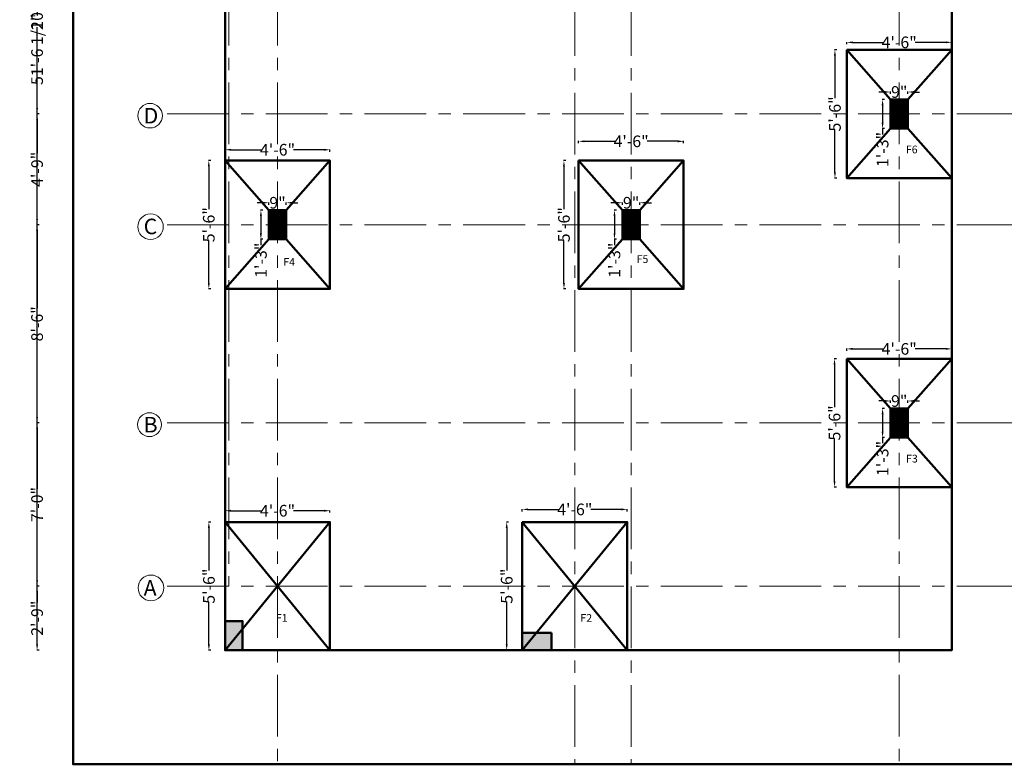
# Model space of a CAD drawing. Units: inches. Extents: x -114 to 953, y -626 to 140.
# Tile 1 of 3: x -114 to 393, y -626 to -243. Entities that reach past the tile are written whole.
import ezdxf

# ---------------------------------------------------------------- set-up
doc = ezdxf.new("R2010")
doc.units = ezdxf.units.IN
doc.header["$MEASUREMENT"] = 0
doc.linetypes.add('CENTER', pattern=[50.8, 31.75, -6.35, 6.35, -6.35])
for name, color, linetype, lineweight in [('S-ANNO-DIMS', 2, 'Continuous', 25), ('S-ANNO-TEXT', 3, 'Continuous', 25), ('S-ANNO-TTLB', 7, 'Continuous', 50), ('S-FNDN', 7, 'Continuous', 50), ('S-FNDN-PATT', 252, 'Continuous', 13), ('S-GRID', 1, 'CENTER', 18), ('S-GRID-IDEN', 7, 'Continuous', 18)]:
    doc.layers.add(name, color=color, linetype=linetype, lineweight=lineweight)
doc.styles.get("Standard").update_dxf_attribs({"font": 'arial.ttf'})
doc.dimstyles.get("Standard").update_dxf_attribs({"dimtxt": 6, "dimasz": 3, "dimexe": 0.18, "dimexo": 0.0625, "dimgap": 0.09, "dimtad": 0, "dimzin": 0, "dimdsep": 46, "dimlunit": 4, "dimtxsty": 'Standard', "dimcen": 0.09, "dimclrd": 256, "dimclrt": 6, "dimadec": 0, "dimazin": 0, "dimtfac": 6, "dimtofl": 0, "dimtmove": 0, "dimatfit": 3, "dimfxl": 1, "dimfxlon": 1, "dimtolj": 1, "dimtzin": 0, "dimarcsym": 0})

# ---------------------------------------------------------------- blocks, each defined once
blk = doc.blocks.new('*D9')
at = {"layer": 'Defpoints', "color": 0, "transparency": 16777216}
for p in [(23.4, -337.38), (14.4, -341.17), (23.4, -341.17)]:
    blk.add_point(p, dxfattribs=at)
at = {"layer": 'S-ANNO-DIMS', "color": 0, "lineweight": -2, "transparency": 16777216}
for p, q in [((11.4, -337.38), (8.4, -337.38)), ((14.4, -338.38), (14.4, -337.2)), ((23.4, -338.38), (23.4, -337.2)), ((26.4, -337.38), (29.4, -337.38))]:
    blk.add_line(p, q, dxfattribs=at)
at = {"layer": 'S-ANNO-DIMS', "color": 0, "transparency": 16777216}
for points in [[(11.4, -336.88), (11.4, -337.88), (14.4, -337.38)], [(26.4, -336.88), (26.4, -337.88), (23.4, -337.38)]]:
    blk.add_solid(points, dxfattribs=at)
at = {"layer": 'S-ANNO-DIMS', "color": 0, "transparency": 16777216, "insert": (18.9, -337.38), "char_height": 6, "attachment_point": 5}
blk.add_mtext('\\A1;9"', dxfattribs=at)
blk = doc.blocks.new('*D10')
at = {"layer": 'Defpoints', "color": 0, "transparency": 16777216}
for p in [(14.4, -341.17), (10.34, -356.17), (14.4, -356.17)]:
    blk.add_point(p, dxfattribs=at)
at = {"layer": 'S-ANNO-DIMS', "color": 0, "lineweight": -2, "transparency": 16777216}
for p, q in [((11.34, -341.17), (10.16, -341.17)), ((10.34, -344.17), (10.34, -353.17)), ((11.34, -356.17), (10.16, -356.17)), ((10.34, -356.17), (10.34, -359.17))]:
    blk.add_line(p, q, dxfattribs=at)
at = {"layer": 'S-ANNO-DIMS', "color": 0, "transparency": 16777216}
for points in [[(9.84, -344.17), (10.84, -344.17), (10.34, -341.17)], [(9.84, -353.17), (10.84, -353.17), (10.34, -356.17)]]:
    blk.add_solid(points, dxfattribs=at)
at = {"layer": 'S-ANNO-DIMS', "color": 0, "transparency": 16777216, "insert": (10.34, -366.95), "char_height": 6, "attachment_point": 5, "rotation": 90}
blk.add_mtext('\\A1;1\'-3"', dxfattribs=at)
blk = doc.blocks.new('*D11')
at = {"layer": 'Defpoints', "color": 0, "transparency": 16777216}
for p in [(343.4, -280.38), (334.4, -284.17), (343.4, -284.17)]:
    blk.add_point(p, dxfattribs=at)
at = {"layer": 'S-ANNO-DIMS', "color": 0, "lineweight": -2, "transparency": 16777216}
for p, q in [((331.4, -280.38), (328.4, -280.38)), ((334.4, -281.38), (334.4, -280.2)), ((343.4, -281.38), (343.4, -280.2)), ((346.4, -280.38), (349.4, -280.38))]:
    blk.add_line(p, q, dxfattribs=at)
at = {"layer": 'S-ANNO-DIMS', "color": 0, "transparency": 16777216}
for points in [[(331.4, -279.88), (331.4, -280.88), (334.4, -280.38)], [(346.4, -279.88), (346.4, -280.88), (343.4, -280.38)]]:
    blk.add_solid(points, dxfattribs=at)
at = {"layer": 'S-ANNO-DIMS', "color": 0, "transparency": 16777216, "insert": (338.9, -280.38), "char_height": 6, "attachment_point": 5}
blk.add_mtext('\\A1;9"', dxfattribs=at)
blk = doc.blocks.new('*D12')
at = {"layer": 'Defpoints', "color": 0, "transparency": 16777216}
for p in [(334.4, -284.17), (330.34, -299.17), (334.4, -299.17)]:
    blk.add_point(p, dxfattribs=at)
at = {"layer": 'S-ANNO-DIMS', "color": 0, "lineweight": -2, "transparency": 16777216}
for p, q in [((331.34, -284.17), (330.16, -284.17)), ((330.34, -287.17), (330.34, -296.17)), ((331.34, -299.17), (330.16, -299.17)), ((330.34, -299.17), (330.34, -302.17))]:
    blk.add_line(p, q, dxfattribs=at)
at = {"layer": 'S-ANNO-DIMS', "color": 0, "transparency": 16777216}
for points in [[(329.84, -287.17), (330.84, -287.17), (330.34, -284.17)], [(329.84, -296.17), (330.84, -296.17), (330.34, -299.17)]]:
    blk.add_solid(points, dxfattribs=at)
at = {"layer": 'S-ANNO-DIMS', "color": 0, "transparency": 16777216, "insert": (330.34, -309.95), "char_height": 6, "attachment_point": 5, "rotation": 90}
blk.add_mtext('\\A1;1\'-3"', dxfattribs=at)
blk = doc.blocks.new('*D13')
at = {"layer": 'Defpoints', "color": 0, "transparency": 16777216}
for p in [(343.4, -439.38), (334.4, -443.17), (343.4, -443.17)]:
    blk.add_point(p, dxfattribs=at)
at = {"layer": 'S-ANNO-DIMS', "color": 0, "lineweight": -2, "transparency": 16777216}
for p, q in [((331.4, -439.38), (328.4, -439.38)), ((334.4, -440.38), (334.4, -439.2)), ((343.4, -440.38), (343.4, -439.2)), ((346.4, -439.38), (349.4, -439.38))]:
    blk.add_line(p, q, dxfattribs=at)
at = {"layer": 'S-ANNO-DIMS', "color": 0, "transparency": 16777216}
for points in [[(331.4, -438.88), (331.4, -439.88), (334.4, -439.38)], [(346.4, -438.88), (346.4, -439.88), (343.4, -439.38)]]:
    blk.add_solid(points, dxfattribs=at)
at = {"layer": 'S-ANNO-DIMS', "color": 0, "transparency": 16777216, "insert": (338.9, -439.38), "char_height": 6, "attachment_point": 5}
blk.add_mtext('\\A1;9"', dxfattribs=at)
blk = doc.blocks.new('*D14')
at = {"layer": 'Defpoints', "color": 0, "transparency": 16777216}
for p in [(334.4, -443.17), (330.34, -458.17), (334.4, -458.17)]:
    blk.add_point(p, dxfattribs=at)
at = {"layer": 'S-ANNO-DIMS', "color": 0, "lineweight": -2, "transparency": 16777216}
for p, q in [((331.34, -443.17), (330.16, -443.17)), ((330.34, -446.17), (330.34, -455.17)), ((331.34, -458.17), (330.16, -458.17)), ((330.34, -458.17), (330.34, -461.17))]:
    blk.add_line(p, q, dxfattribs=at)
at = {"layer": 'S-ANNO-DIMS', "color": 0, "transparency": 16777216}
for points in [[(329.84, -446.17), (330.84, -446.17), (330.34, -443.17)], [(329.84, -455.17), (330.84, -455.17), (330.34, -458.17)]]:
    blk.add_solid(points, dxfattribs=at)
at = {"layer": 'S-ANNO-DIMS', "color": 0, "transparency": 16777216, "insert": (330.34, -468.95), "char_height": 6, "attachment_point": 5, "rotation": 90}
blk.add_mtext('\\A1;1\'-3"', dxfattribs=at)
blk = doc.blocks.new('*D19')
at = {"layer": 'Defpoints', "color": 0, "transparency": 16777216}
for p in [(205.4, -337.38), (196.4, -341.17), (205.4, -341.17)]:
    blk.add_point(p, dxfattribs=at)
at = {"layer": 'S-ANNO-DIMS', "color": 0, "lineweight": -2, "transparency": 16777216}
for p, q in [((193.4, -337.38), (190.4, -337.38)), ((196.4, -338.38), (196.4, -337.2)), ((205.4, -338.38), (205.4, -337.2)), ((208.4, -337.38), (211.4, -337.38))]:
    blk.add_line(p, q, dxfattribs=at)
at = {"layer": 'S-ANNO-DIMS', "color": 0, "transparency": 16777216}
for points in [[(193.4, -336.88), (193.4, -337.88), (196.4, -337.38)], [(208.4, -336.88), (208.4, -337.88), (205.4, -337.38)]]:
    blk.add_solid(points, dxfattribs=at)
at = {"layer": 'S-ANNO-DIMS', "color": 0, "transparency": 16777216, "insert": (200.9, -337.38), "char_height": 6, "attachment_point": 5}
blk.add_mtext('\\A1;9"', dxfattribs=at)
blk = doc.blocks.new('*D20')
at = {"layer": 'Defpoints', "color": 0, "transparency": 16777216}
for p in [(196.4, -341.17), (192.33, -356.17), (196.4, -356.17)]:
    blk.add_point(p, dxfattribs=at)
at = {"layer": 'S-ANNO-DIMS', "color": 0, "lineweight": -2, "transparency": 16777216}
for p, q in [((193.33, -341.17), (192.15, -341.17)), ((192.33, -344.17), (192.33, -353.17)), ((193.33, -356.17), (192.15, -356.17)), ((192.33, -356.17), (192.33, -359.17))]:
    blk.add_line(p, q, dxfattribs=at)
at = {"layer": 'S-ANNO-DIMS', "color": 0, "transparency": 16777216}
for points in [[(191.83, -344.17), (192.83, -344.17), (192.33, -341.17)], [(191.83, -353.17), (192.83, -353.17), (192.33, -356.17)]]:
    blk.add_solid(points, dxfattribs=at)
at = {"layer": 'S-ANNO-DIMS', "color": 0, "transparency": 16777216, "insert": (192.33, -366.95), "char_height": 6, "attachment_point": 5, "rotation": 90}
blk.add_mtext('\\A1;1\'-3"', dxfattribs=at)
blk = doc.blocks.new('*D33')
at = {"layer": 'Defpoints', "color": 0, "transparency": 16777216}
for p in [(45.9, -310.1), (-8.1, -315.67), (45.9, -315.67)]:
    blk.add_point(p, dxfattribs=at)
at = {"layer": 'S-ANNO-DIMS', "color": 0, "lineweight": -2, "transparency": 16777216}
for p, q in [((-8.1, -311.1), (-8.1, -309.92)), ((-5.1, -310.1), (10.72, -310.1)), ((42.9, -310.1), (27.09, -310.1)), ((45.9, -311.1), (45.9, -309.92))]:
    blk.add_line(p, q, dxfattribs=at)
at = {"layer": 'S-ANNO-DIMS', "color": 0, "transparency": 16777216}
for points in [[(-5.1, -309.6), (-5.1, -310.6), (-8.1, -310.1)], [(42.9, -309.6), (42.9, -310.6), (45.9, -310.1)]]:
    blk.add_solid(points, dxfattribs=at)
at = {"layer": 'S-ANNO-DIMS', "color": 0, "transparency": 16777216, "insert": (18.9, -310.1), "char_height": 6, "attachment_point": 5}
blk.add_mtext('\\A1;4\'-6"', dxfattribs=at)
blk = doc.blocks.new('*D34')
at = {"layer": 'Defpoints', "color": 0, "transparency": 16777216}
for p in [(-8.1, -315.67), (-16.48, -381.67), (-8.1, -381.67)]:
    blk.add_point(p, dxfattribs=at)
at = {"layer": 'S-ANNO-DIMS', "color": 0, "lineweight": -2, "transparency": 16777216}
for p, q in [((-15.48, -315.67), (-16.66, -315.67)), ((-16.48, -318.67), (-16.48, -340.6)), ((-16.48, -378.67), (-16.48, -356.73)), ((-15.48, -381.67), (-16.66, -381.67))]:
    blk.add_line(p, q, dxfattribs=at)
at = {"layer": 'S-ANNO-DIMS', "color": 0, "transparency": 16777216}
for points in [[(-16.98, -318.67), (-15.98, -318.67), (-16.48, -315.67)], [(-16.98, -378.67), (-15.98, -378.67), (-16.48, -381.67)]]:
    blk.add_solid(points, dxfattribs=at)
at = {"layer": 'S-ANNO-DIMS', "color": 0, "transparency": 16777216, "insert": (-16.48, -348.67), "char_height": 6, "attachment_point": 5, "rotation": 90}
blk.add_mtext('\\A1;5\'-6"', dxfattribs=at)
blk = doc.blocks.new('*D35')
at = {"layer": 'Defpoints', "color": 0, "transparency": 16777216}
for p in [(227.9, -305.76), (173.9, -315.67), (227.9, -315.67)]:
    blk.add_point(p, dxfattribs=at)
at = {"layer": 'S-ANNO-DIMS', "color": 0, "lineweight": -2, "transparency": 16777216}
for p, q in [((173.9, -306.76), (173.9, -305.58)), ((176.9, -305.76), (192.71, -305.76)), ((224.9, -305.76), (209.08, -305.76)), ((227.9, -306.76), (227.9, -305.58))]:
    blk.add_line(p, q, dxfattribs=at)
at = {"layer": 'S-ANNO-DIMS', "color": 0, "transparency": 16777216}
for points in [[(176.9, -305.26), (176.9, -306.26), (173.9, -305.76)], [(224.9, -305.26), (224.9, -306.26), (227.9, -305.76)]]:
    blk.add_solid(points, dxfattribs=at)
at = {"layer": 'S-ANNO-DIMS', "color": 0, "transparency": 16777216, "insert": (200.9, -305.76), "char_height": 6, "attachment_point": 5}
blk.add_mtext('\\A1;4\'-6"', dxfattribs=at)
blk = doc.blocks.new('*D36')
at = {"layer": 'Defpoints', "color": 0, "transparency": 16777216}
for p in [(173.9, -315.67), (166.33, -381.67), (173.9, -381.67)]:
    blk.add_point(p, dxfattribs=at)
at = {"layer": 'S-ANNO-DIMS', "color": 0, "lineweight": -2, "transparency": 16777216}
for p, q in [((167.33, -315.67), (166.15, -315.67)), ((166.33, -318.67), (166.33, -340.6)), ((166.33, -378.67), (166.33, -356.73)), ((167.33, -381.67), (166.15, -381.67))]:
    blk.add_line(p, q, dxfattribs=at)
at = {"layer": 'S-ANNO-DIMS', "color": 0, "transparency": 16777216}
for points in [[(165.83, -318.67), (166.83, -318.67), (166.33, -315.67)], [(165.83, -378.67), (166.83, -378.67), (166.33, -381.67)]]:
    blk.add_solid(points, dxfattribs=at)
at = {"layer": 'S-ANNO-DIMS', "color": 0, "transparency": 16777216, "insert": (166.33, -348.67), "char_height": 6, "attachment_point": 5, "rotation": 90}
blk.add_mtext('\\A1;5\'-6"', dxfattribs=at)
blk = doc.blocks.new('*D37')
at = {"layer": 'Defpoints', "color": 0, "transparency": 16777216}
for p in [(365.9, -254.83), (311.9, -258.67), (365.9, -258.67)]:
    blk.add_point(p, dxfattribs=at)
at = {"layer": 'S-ANNO-DIMS', "color": 0, "lineweight": -2, "transparency": 16777216}
for p, q in [((311.9, -255.83), (311.9, -254.65)), ((314.9, -254.83), (330.72, -254.83)), ((362.9, -254.83), (347.09, -254.83)), ((365.9, -255.83), (365.9, -254.65))]:
    blk.add_line(p, q, dxfattribs=at)
at = {"layer": 'S-ANNO-DIMS', "color": 0, "transparency": 16777216}
for points in [[(314.9, -254.33), (314.9, -255.33), (311.9, -254.83)], [(362.9, -254.33), (362.9, -255.33), (365.9, -254.83)]]:
    blk.add_solid(points, dxfattribs=at)
at = {"layer": 'S-ANNO-DIMS', "color": 0, "transparency": 16777216, "insert": (338.9, -254.83), "char_height": 6, "attachment_point": 5}
blk.add_mtext('\\A1;4\'-6"', dxfattribs=at)
blk = doc.blocks.new('*D38')
at = {"layer": 'Defpoints', "color": 0, "transparency": 16777216}
for p in [(311.9, -258.67), (305.81, -324.67), (311.9, -324.67)]:
    blk.add_point(p, dxfattribs=at)
at = {"layer": 'S-ANNO-DIMS', "color": 0, "lineweight": -2, "transparency": 16777216}
for p, q in [((306.81, -258.67), (305.63, -258.67)), ((305.81, -261.67), (305.81, -283.6)), ((305.81, -321.67), (305.81, -299.73)), ((306.81, -324.67), (305.63, -324.67))]:
    blk.add_line(p, q, dxfattribs=at)
at = {"layer": 'S-ANNO-DIMS', "color": 0, "transparency": 16777216}
for points in [[(305.31, -261.67), (306.31, -261.67), (305.81, -258.67)], [(305.31, -321.67), (306.31, -321.67), (305.81, -324.67)]]:
    blk.add_solid(points, dxfattribs=at)
at = {"layer": 'S-ANNO-DIMS', "color": 0, "transparency": 16777216, "insert": (305.81, -291.67), "char_height": 6, "attachment_point": 5, "rotation": 90}
blk.add_mtext('\\A1;5\'-6"', dxfattribs=at)
blk = doc.blocks.new('*D39')
at = {"layer": 'Defpoints', "color": 0, "transparency": 16777216}
for p in [(-8.1, -495.85), (-8.1, -501.67), (45.9, -501.67)]:
    blk.add_point(p, dxfattribs=at)
at = {"layer": 'S-ANNO-DIMS', "color": 0, "lineweight": -2, "transparency": 16777216}
for p, q in [((-8.1, -496.85), (-8.1, -495.67)), ((-5.1, -495.85), (10.72, -495.85)), ((42.9, -495.85), (27.09, -495.85)), ((45.9, -496.85), (45.9, -495.67))]:
    blk.add_line(p, q, dxfattribs=at)
at = {"layer": 'S-ANNO-DIMS', "color": 0, "transparency": 16777216}
for points in [[(-5.1, -495.35), (-5.1, -496.35), (-8.1, -495.85)], [(42.9, -495.35), (42.9, -496.35), (45.9, -495.85)]]:
    blk.add_solid(points, dxfattribs=at)
at = {"layer": 'S-ANNO-DIMS', "color": 0, "transparency": 16777216, "insert": (18.9, -495.85), "char_height": 6, "attachment_point": 5}
blk.add_mtext('\\A1;4\'-6"', dxfattribs=at)
blk = doc.blocks.new('*D40')
at = {"layer": 'Defpoints', "color": 0, "transparency": 16777216}
for p in [(-8.1, -501.67), (-16.43, -567.67), (-8.1, -567.67)]:
    blk.add_point(p, dxfattribs=at)
at = {"layer": 'S-ANNO-DIMS', "color": 0, "lineweight": -2, "transparency": 16777216}
for p, q in [((-15.43, -501.67), (-16.61, -501.67)), ((-16.43, -504.67), (-16.43, -526.6)), ((-16.43, -564.67), (-16.43, -542.73)), ((-15.43, -567.67), (-16.61, -567.67))]:
    blk.add_line(p, q, dxfattribs=at)
at = {"layer": 'S-ANNO-DIMS', "color": 0, "transparency": 16777216}
for points in [[(-16.93, -504.67), (-15.93, -504.67), (-16.43, -501.67)], [(-16.93, -564.67), (-15.93, -564.67), (-16.43, -567.67)]]:
    blk.add_solid(points, dxfattribs=at)
at = {"layer": 'S-ANNO-DIMS', "color": 0, "transparency": 16777216, "insert": (-16.43, -534.67), "char_height": 6, "attachment_point": 5, "rotation": 90}
blk.add_mtext('\\A1;5\'-6"', dxfattribs=at)
blk = doc.blocks.new('*D41')
at = {"layer": 'Defpoints', "color": 0, "transparency": 16777216}
for p in [(144.9, -495.18), (144.9, -501.67), (198.9, -501.67)]:
    blk.add_point(p, dxfattribs=at)
at = {"layer": 'S-ANNO-DIMS', "color": 0, "lineweight": -2, "transparency": 16777216}
for p, q in [((144.9, -496.18), (144.9, -495)), ((147.9, -495.18), (163.71, -495.18)), ((195.9, -495.18), (180.08, -495.18)), ((198.9, -496.18), (198.9, -495))]:
    blk.add_line(p, q, dxfattribs=at)
at = {"layer": 'S-ANNO-DIMS', "color": 0, "transparency": 16777216}
for points in [[(147.9, -494.68), (147.9, -495.68), (144.9, -495.18)], [(195.9, -494.68), (195.9, -495.68), (198.9, -495.18)]]:
    blk.add_solid(points, dxfattribs=at)
at = {"layer": 'S-ANNO-DIMS', "color": 0, "transparency": 16777216, "insert": (171.9, -495.18), "char_height": 6, "attachment_point": 5}
blk.add_mtext('\\A1;4\'-6"', dxfattribs=at)
blk = doc.blocks.new('*D42')
at = {"layer": 'Defpoints', "color": 0, "transparency": 16777216}
for p in [(144.9, -501.67), (136.86, -567.67), (144.9, -567.67)]:
    blk.add_point(p, dxfattribs=at)
at = {"layer": 'S-ANNO-DIMS', "color": 0, "lineweight": -2, "transparency": 16777216}
for p, q in [((137.86, -501.67), (136.68, -501.67)), ((136.86, -504.67), (136.86, -526.6)), ((136.86, -564.67), (136.86, -542.73)), ((137.86, -567.67), (136.68, -567.67))]:
    blk.add_line(p, q, dxfattribs=at)
at = {"layer": 'S-ANNO-DIMS', "color": 0, "transparency": 16777216}
for points in [[(136.36, -504.67), (137.36, -504.67), (136.86, -501.67)], [(136.36, -564.67), (137.36, -564.67), (136.86, -567.67)]]:
    blk.add_solid(points, dxfattribs=at)
at = {"layer": 'S-ANNO-DIMS', "color": 0, "transparency": 16777216, "insert": (136.86, -534.67), "char_height": 6, "attachment_point": 5, "rotation": 90}
blk.add_mtext('\\A1;5\'-6"', dxfattribs=at)
blk = doc.blocks.new('*D43')
at = {"layer": 'Defpoints', "color": 0, "transparency": 16777216}
for p in [(311.9, -412.58), (311.9, -417.67), (365.9, -417.67)]:
    blk.add_point(p, dxfattribs=at)
at = {"layer": 'S-ANNO-DIMS', "color": 0, "lineweight": -2, "transparency": 16777216}
for p, q in [((311.9, -413.58), (311.9, -412.4)), ((314.9, -412.58), (330.72, -412.58)), ((362.9, -412.58), (347.09, -412.58)), ((365.9, -413.58), (365.9, -412.4))]:
    blk.add_line(p, q, dxfattribs=at)
at = {"layer": 'S-ANNO-DIMS', "color": 0, "transparency": 16777216}
for points in [[(314.9, -412.08), (314.9, -413.08), (311.9, -412.58)], [(362.9, -412.08), (362.9, -413.08), (365.9, -412.58)]]:
    blk.add_solid(points, dxfattribs=at)
at = {"layer": 'S-ANNO-DIMS', "color": 0, "transparency": 16777216, "insert": (338.9, -412.58), "char_height": 6, "attachment_point": 5}
blk.add_mtext('\\A1;4\'-6"', dxfattribs=at)
blk = doc.blocks.new('*D44')
at = {"layer": 'Defpoints', "color": 0, "transparency": 16777216}
for p in [(311.9, -417.67), (305.61, -483.67), (311.9, -483.67)]:
    blk.add_point(p, dxfattribs=at)
at = {"layer": 'S-ANNO-DIMS', "color": 0, "lineweight": -2, "transparency": 16777216}
for p, q in [((306.61, -417.67), (305.43, -417.67)), ((305.61, -420.67), (305.61, -442.6)), ((305.61, -480.67), (305.61, -458.73)), ((306.61, -483.67), (305.43, -483.67))]:
    blk.add_line(p, q, dxfattribs=at)
at = {"layer": 'S-ANNO-DIMS', "color": 0, "transparency": 16777216}
for points in [[(305.11, -420.67), (306.11, -420.67), (305.61, -417.67)], [(305.11, -480.67), (306.11, -480.67), (305.61, -483.67)]]:
    blk.add_solid(points, dxfattribs=at)
at = {"layer": 'S-ANNO-DIMS', "color": 0, "transparency": 16777216, "insert": (305.61, -450.67), "char_height": 6, "attachment_point": 5, "rotation": 90}
blk.add_mtext('\\A1;5\'-6"', dxfattribs=at)
blk = doc.blocks.new('FOOTING-ISOL-COL')
h = blk.add_hatch()
h.set_pattern_fill('2X2µØ×©', color=256)
h.set_pattern_definition([(0, (379.9615, 68.9256), (0.5, 0.5), [0.45, -0.05, 0.2, -0.05, 0.2, -0.05]), (0, (379.9615, 69.1256), (0.5, 0.5), [0.45, -0.55]), (0, (379.9615, 69.1756), (0.5, 0.5), [0.45, -0.55]), (0, (379.9615, 69.3756), (0.5, 0.5), [0.45, -0.05, 0.2, -0.05, 0.2, -0.05]), (90, (379.9615, 68.9256), (-0.5, 0.5), [0.2, -0.05, 0.2, -0.05, 0.45, -0.05]), (90, (380.4115, 68.9256), (-0.5, 0.5), [0.2, -0.05, 0.2, -0.05, 0.45, -0.05]), (90, (380.6615, 68.9256), (-0.5, 0.5), [0.45, -0.55]), (90, (380.7115, 68.9256), (-0.5, 0.5), [0.45, -0.55])])
h.paths.add_polyline_path([(23.4, 10.33), (14.4, 10.33), (14.4, -4.67), (23.4, -4.67)])
for p, q in [((14.4, 10.33), (-8.1, 35.83)), ((23.4, 10.33), (45.9, 35.83)), ((14.4, -4.67), (-8.1, -30.17)), ((23.4, -4.67), (45.9, -30.17))]:
    blk.add_line(p, q)
for points in [[(-8.1, 35.83), (45.9, 35.83), (45.9, -30.17), (-8.1, -30.17)], [(14.4, 10.33), (23.4, 10.33), (23.4, -4.67), (14.4, -4.67)]]:
    blk.add_lwpolyline(points, close=True)
blk = doc.blocks.new('FOOTING-CORNER')
for p, q in [((-8.1, -501.67), (45.9, -567.67)), ((-8.1, -567.67), (45.9, -501.67))]:
    blk.add_line(p, q)
blk.add_lwpolyline([(-8.1, -501.67), (45.9, -501.67), (45.9, -567.67), (-8.1, -567.67)], close=True)
blk = doc.blocks.new('*D57')
at = {"layer": 'Defpoints', "color": 0, "transparency": 16777216}
for p in [(-37.87, -168.17), (-104.87, -291.67), (-37.87, -291.67)]:
    blk.add_point(p, dxfattribs=at)
at = {"layer": 'S-ANNO-DIMS', "color": 0, "lineweight": -2, "transparency": 16777216}
for p, q in [((-103.87, -168.17), (-105.05, -168.17)), ((-103.87, -291.67), (-105.05, -291.67))]:
    blk.add_line(p, q, dxfattribs=at)
at = {"layer": 'S-ANNO-DIMS', "lineweight": -2, "transparency": 16777216}
for p, q in [((-104.87, -171.17), (-104.87, -212.81)), ((-104.87, -288.67), (-104.87, -247.02))]:
    blk.add_line(p, q, dxfattribs=at)
at = {"layer": 'S-ANNO-DIMS', "transparency": 16777216}
for points in [[(-105.37, -171.17), (-104.37, -171.17), (-104.87, -168.17)], [(-105.37, -288.67), (-104.37, -288.67), (-104.87, -291.67)]]:
    blk.add_solid(points, dxfattribs=at)
at = {"layer": 'S-ANNO-DIMS', "color": 6, "transparency": 16777216, "insert": (-104.87, -229.92), "char_height": 6, "attachment_point": 5, "rotation": 90}
blk.add_mtext('\\A1;10\'-3 1/2"', dxfattribs=at)
blk = doc.blocks.new('*D58')
at = {"layer": 'Defpoints', "color": 0, "transparency": 16777216}
for p in [(-37.87, -291.67), (-104.87, -348.67), (-37.87, -348.67)]:
    blk.add_point(p, dxfattribs=at)
at = {"layer": 'S-ANNO-DIMS', "color": 0, "lineweight": -2, "transparency": 16777216}
for p, q in [((-103.87, -291.67), (-105.05, -291.67)), ((-103.87, -348.67), (-105.05, -348.67))]:
    blk.add_line(p, q, dxfattribs=at)
at = {"layer": 'S-ANNO-DIMS', "lineweight": -2, "transparency": 16777216}
for p, q in [((-104.87, -294.67), (-104.87, -311.98)), ((-104.87, -345.67), (-104.87, -328.35))]:
    blk.add_line(p, q, dxfattribs=at)
at = {"layer": 'S-ANNO-DIMS', "transparency": 16777216}
for points in [[(-105.37, -294.67), (-104.37, -294.67), (-104.87, -291.67)], [(-105.37, -345.67), (-104.37, -345.67), (-104.87, -348.67)]]:
    blk.add_solid(points, dxfattribs=at)
at = {"layer": 'S-ANNO-DIMS', "color": 6, "transparency": 16777216, "insert": (-104.87, -320.17), "char_height": 6, "attachment_point": 5, "rotation": 90}
blk.add_mtext('\\A1;4\'-9"', dxfattribs=at)
blk = doc.blocks.new('*D59')
at = {"layer": 'Defpoints', "color": 0, "transparency": 16777216}
for p in [(-37.87, -348.67), (-104.87, -450.67), (-37.87, -450.67)]:
    blk.add_point(p, dxfattribs=at)
at = {"layer": 'S-ANNO-DIMS', "color": 0, "lineweight": -2, "transparency": 16777216}
for p, q in [((-103.87, -348.67), (-105.05, -348.67)), ((-103.87, -450.67), (-105.05, -450.67))]:
    blk.add_line(p, q, dxfattribs=at)
at = {"layer": 'S-ANNO-DIMS', "lineweight": -2, "transparency": 16777216}
for p, q in [((-104.87, -351.67), (-104.87, -391.6)), ((-104.87, -447.67), (-104.87, -407.74))]:
    blk.add_line(p, q, dxfattribs=at)
at = {"layer": 'S-ANNO-DIMS', "transparency": 16777216}
for points in [[(-105.37, -351.67), (-104.37, -351.67), (-104.87, -348.67)], [(-105.37, -447.67), (-104.37, -447.67), (-104.87, -450.67)]]:
    blk.add_solid(points, dxfattribs=at)
at = {"layer": 'S-ANNO-DIMS', "color": 6, "transparency": 16777216, "insert": (-104.87, -399.67), "char_height": 6, "attachment_point": 5, "rotation": 90}
blk.add_mtext('\\A1;8\'-6"', dxfattribs=at)
blk = doc.blocks.new('*D60')
at = {"layer": 'Defpoints', "color": 0, "transparency": 16777216}
for p in [(-37.87, -450.67), (-104.87, -534.67), (-37.87, -534.67)]:
    blk.add_point(p, dxfattribs=at)
at = {"layer": 'S-ANNO-DIMS', "color": 0, "lineweight": -2, "transparency": 16777216}
for p, q in [((-103.87, -450.67), (-105.05, -450.67)), ((-103.87, -534.67), (-105.05, -534.67))]:
    blk.add_line(p, q, dxfattribs=at)
at = {"layer": 'S-ANNO-DIMS', "lineweight": -2, "transparency": 16777216}
for p, q in [((-104.87, -453.67), (-104.87, -484.63)), ((-104.87, -531.67), (-104.87, -500.71))]:
    blk.add_line(p, q, dxfattribs=at)
at = {"layer": 'S-ANNO-DIMS', "transparency": 16777216}
for points in [[(-105.37, -453.67), (-104.37, -453.67), (-104.87, -450.67)], [(-105.37, -531.67), (-104.37, -531.67), (-104.87, -534.67)]]:
    blk.add_solid(points, dxfattribs=at)
at = {"layer": 'S-ANNO-DIMS', "color": 6, "transparency": 16777216, "insert": (-104.87, -492.67), "char_height": 6, "attachment_point": 5, "rotation": 90}
blk.add_mtext('\\A1;7\'-0"', dxfattribs=at)
blk = doc.blocks.new('*D62')
at = {"layer": 'Defpoints', "color": 0, "transparency": 16777216}
for p in [(-37.87, -534.67), (-104.87, -567.67), (-8.1, -567.67)]:
    blk.add_point(p, dxfattribs=at)
at = {"layer": 'S-ANNO-DIMS', "color": 0, "lineweight": -2, "transparency": 16777216}
for p, q in [((-103.87, -534.67), (-105.05, -534.67)), ((-103.87, -567.67), (-105.05, -567.67))]:
    blk.add_line(p, q, dxfattribs=at)
at = {"layer": 'S-ANNO-DIMS', "lineweight": -2, "transparency": 16777216}
for p, q in [((-104.87, -537.67), (-104.87, -543.05)), ((-104.87, -564.67), (-104.87, -559.28))]:
    blk.add_line(p, q, dxfattribs=at)
at = {"layer": 'S-ANNO-DIMS', "transparency": 16777216}
for points in [[(-105.37, -537.67), (-104.37, -537.67), (-104.87, -534.67)], [(-105.37, -564.67), (-104.37, -564.67), (-104.87, -567.67)]]:
    blk.add_solid(points, dxfattribs=at)
at = {"layer": 'S-ANNO-DIMS', "color": 6, "transparency": 16777216, "insert": (-104.87, -551.17), "char_height": 6, "attachment_point": 5, "rotation": 90}
blk.add_mtext('\\A1;2\'-9"', dxfattribs=at)
blk = doc.blocks.new('*D63')
at = {"layer": 'Defpoints', "color": 0, "transparency": 16777216}
for p in [(-8.1, 50.84), (-104.87, -567.67), (-8.1, -567.67)]:
    blk.add_point(p, dxfattribs=at)
at = {"layer": 'S-ANNO-DIMS', "color": 0, "lineweight": -2, "transparency": 16777216}
for p, q in [((-103.87, 50.84), (-105.05, 50.84)), ((-103.87, -567.67), (-105.05, -567.67))]:
    blk.add_line(p, q, dxfattribs=at)
at = {"layer": 'S-ANNO-DIMS', "lineweight": -2, "transparency": 16777216}
for p, q in [((-104.87, 47.84), (-104.87, -241.03)), ((-104.87, -564.67), (-104.87, -275.8))]:
    blk.add_line(p, q, dxfattribs=at)
at = {"layer": 'S-ANNO-DIMS', "transparency": 16777216}
for points in [[(-105.37, 47.84), (-104.37, 47.84), (-104.87, 50.84)], [(-105.37, -564.67), (-104.37, -564.67), (-104.87, -567.67)]]:
    blk.add_solid(points, dxfattribs=at)
at = {"layer": 'S-ANNO-DIMS', "color": 6, "transparency": 16777216, "insert": (-104.87, -258.41), "char_height": 6, "attachment_point": 5, "rotation": 90}
blk.add_mtext('\\A1;51\'-6 1/2"', dxfattribs=at)

msp = doc.modelspace()

# ---------------------------------------------------------------- hatches: boundary and pattern name
at = {"layer": 'S-FNDN-PATT'}
h = msp.add_hatch(dxfattribs=at)
h.set_pattern_fill('2X2µØ×©', color=256)
h.set_pattern_definition([(0, (0, 0), (0.5, 0.5), [0.45, -0.05, 0.2, -0.05, 0.2, -0.05]), (0, (0, 0.2), (0.5, 0.5), [0.45, -0.55]), (0, (0, 0.25), (0.5, 0.5), [0.45, -0.55]), (0, (0, 0.45), (0.5, 0.5), [0.45, -0.05, 0.2, -0.05, 0.2, -0.05]), (90, (0, 0), (-0.5, 0.5), [0.2, -0.05, 0.2, -0.05, 0.45, -0.05]), (90, (0.45, 0), (-0.5, 0.5), [0.2, -0.05, 0.2, -0.05, 0.45, -0.05]), (90, (0.7, 0), (-0.5, 0.5), [0.45, -0.55]), (90, (0.75, 0), (-0.5, 0.5), [0.45, -0.55])])
h.paths.add_polyline_path([(0.902, -552.669), (-8.098, -552.669), (-8.098, -567.669), (0.902, -556.669)])
h.paths.add_polyline_path([(0.902, -556.669), (-8.098, -567.669), (0.902, -567.669)])
h.paths.add_polyline_path([(159.897, -558.669), (152.261, -558.669), (144.897, -567.669), (159.897, -567.669)])
h.paths.add_polyline_path([(152.261, -558.669), (144.897, -558.669), (144.897, -567.669)])

# ---------------------------------------------------------------- linework, layer by layer
at = {"layer": 'S-ANNO-TTLB'}
msp.add_lwpolyline([(-86.343, 140.009), (953.065, 140.009), (953.065, -626.35), (-86.343, -626.35)], close=True, dxfattribs=at)
at = {"layer": 'S-FNDN'}
for points in [[(-8.098, 50.843), (365.902, 50.843), (365.902, -567.669), (-8.098, -567.669)], [(-8.098, -552.669), (0.902, -552.669), (0.902, -567.669), (-8.098, -567.669)], [(159.897, -558.669), (159.897, -567.669), (144.897, -567.669), (144.897, -558.669)]]:
    msp.add_lwpolyline(points, close=True, dxfattribs=at)
at = {"layer": 'S-GRID'}
for p, q in [((-6.098, 80.047), (-6.098, -534.669)), ((18.902, 80.047), (18.902, -626.35)), ((338.902, 80.047), (338.902, -626.35)), ((171.897, 74.831), (171.897, -626.35)), ((200.897, 74.831), (200.897, -626.35)), ((-37.867, -291.669), (403.662, -291.669)), ((-37.867, -348.669), (403.662, -348.669)), ((-37.867, -450.669), (403.662, -450.669)), ((-37.867, -534.669), (403.662, -534.669))]:
    msp.add_line(p, q, dxfattribs=at)
at = {"layer": 'S-GRID-IDEN'}
for centre, radius in [((-46.691, -292.569), 6.317), ((-46.461, -349.705), 6.57), ((-46.977, -451.569), 6.135), ((-46.262, -535.569), 6.604)]:
    msp.add_circle(centre, radius, dxfattribs=at)

# ---------------------------------------------------------------- block references
at = {"layer": 'S-FNDN'}
for name, p in [('FOOTING-ISOL-COL', (320, -294.5)), ('FOOTING-ISOL-COL', (0, -351.5)), ('FOOTING-ISOL-COL', (181.996, -351.5)), ('FOOTING-ISOL-COL', (320, -453.5)), ('FOOTING-CORNER', (0, 0)), ('FOOTING-CORNER', (152.996, 0))]:
    msp.add_blockref(name, p, dxfattribs=at)

# ---------------------------------------------------------------- texts
at = {"layer": 'S-ANNO-TEXT', "char_height": 4, "attachment_point": 1}
for s, insert in [('{\\fArial|b1|i0|c0|p34;F6}', (342.344, -307.955)), ('{\\fArial|b1|i0|c0|p34;F5}', (203.735, -364.369)), ('{\\fArial|b1|i0|c0|p34;F4}', (21.886, -365.821)), ('{\\fArial|b1|i0|c0|p34;F3}', (342.419, -467.044)), ('{\\fArial|b1|i0|c0|p34;F1}', (18.055, -549.016)), ('{\\fArial|b1|i0|c0|p34;F2}', (174.792, -549.016))]:
    msp.add_mtext_dynamic_manual_height_columns(s, width=16.75606, gutter_width=1, heights=[0], dxfattribs=dict(at, insert=insert))
at = {"layer": 'S-GRID-IDEN', "char_height": 8, "attachment_point": 1}
for s, insert in [('D', (-49.998, -288.569)), ('C', (-49.998, -345.569)), ('B', (-49.998, -447.569)), ('A', (-49.998, -531.569))]:
    msp.add_mtext_dynamic_manual_height_columns(s, width=16.75606, gutter_width=1, heights=[0], dxfattribs=dict(at, insert=insert))

# ---------------------------------------------------------------- dimensions: what is measured, and where the dimension line sits
at = {"layer": 'S-ANNO-DIMS'}
for base, p1, p2, override, picture, middle in [((-104.87, -567.669), (-8.098, 50.843), (-8.098, -567.669), {"dimdec": 1, "dimlfac": 1, "dimrnd": 0, "dimzin": 1, "dimdsep": 46, "dimlunit": 4, "dimfrac": 2}, '*D63', (-104.87, -258.413)), ((-104.87, -291.669), (-37.867, -168.169), (-37.867, -291.669), {"dimdec": 1, "dimlfac": 1, "dimrnd": 0, "dimzin": 1, "dimdsep": 46, "dimlunit": 4, "dimfrac": 2}, '*D57', (-104.87, -229.919)), ((305.806, -324.669), (311.902, -258.669), (311.902, -324.669), {"dimclrd": 0, "dimclre": 0, "dimclrt": 0}, '*D38', (305.806, -291.669)), ((330.338, -299.169), (334.402, -284.169), (334.402, -299.169), {"dimclrd": 0, "dimclre": 0, "dimclrt": 0}, '*D12', (330.338, -309.951)), ((-104.87, -348.669), (-37.867, -291.669), (-37.867, -348.669), {"dimdec": 1, "dimlfac": 1, "dimrnd": 0, "dimzin": 1, "dimdsep": 46, "dimlunit": 4, "dimfrac": 2}, '*D58', (-104.87, -320.169)), ((-16.484, -381.669), (-8.098, -315.669), (-8.098, -381.669), {"dimclrd": 0, "dimclre": 0, "dimclrt": 0}, '*D34', (-16.484, -348.669)), ((166.332, -381.669), (173.897, -315.669), (173.897, -381.669), {"dimclrd": 0, "dimclre": 0, "dimclrt": 0}, '*D36', (166.332, -348.669)), ((10.338, -356.169), (14.402, -341.169), (14.402, -356.169), {"dimclrd": 0, "dimclre": 0, "dimclrt": 0}, '*D10', (10.338, -366.951)), ((192.334, -356.169), (196.397, -341.169), (196.397, -356.169), {"dimclrd": 0, "dimclre": 0, "dimclrt": 0}, '*D20', (192.334, -366.951)), ((-104.87, -450.669), (-37.867, -348.669), (-37.867, -450.669), {"dimdec": 1, "dimlfac": 1, "dimrnd": 0, "dimzin": 1, "dimdsep": 46, "dimlunit": 4, "dimfrac": 2}, '*D59', (-104.87, -399.669)), ((305.609, -483.669), (311.902, -417.669), (311.902, -483.669), {"dimclrd": 0, "dimclre": 0, "dimclrt": 0}, '*D44', (305.609, -450.669)), ((330.338, -458.169), (334.402, -443.169), (334.402, -458.169), {"dimclrd": 0, "dimclre": 0, "dimclrt": 0}, '*D14', (330.338, -468.951)), ((-104.87, -534.669), (-37.867, -450.669), (-37.867, -534.669), {"dimdec": 1, "dimlfac": 1, "dimrnd": 0, "dimzin": 1, "dimdsep": 46, "dimlunit": 4, "dimfrac": 2}, '*D60', (-104.87, -492.669)), ((-16.428, -567.669), (-8.098, -501.669), (-8.098, -567.669), {"dimclrd": 0, "dimclre": 0, "dimclrt": 0}, '*D40', (-16.428, -534.669)), ((136.863, -567.669), (144.897, -501.669), (144.897, -567.669), {"dimclrd": 0, "dimclre": 0, "dimclrt": 0}, '*D42', (136.863, -534.669)), ((-104.87, -567.669), (-37.867, -534.669), (-8.098, -567.669), {"dimdec": 1, "dimlfac": 1, "dimrnd": 0, "dimzin": 1, "dimdsep": 46, "dimlunit": 4, "dimfrac": 2}, '*D62', (-104.87, -551.169))]:
    dim = msp.add_linear_dim(base=base, p1=p1, p2=p2, angle=90, dimstyle='Standard', override=override, dxfattribs=at)
    dim.commit()
    dim.dimension.update_dxf_attribs({"geometry": picture, "text_midpoint": middle})
for base, p1, p2, picture, middle in [((365.902, -254.828), (311.902, -258.669), (365.902, -258.669), '*D37', (338.902, -254.828)), ((343.402, -280.375), (334.402, -284.169), (343.402, -284.169), '*D11', (338.902, -280.375)), ((227.897, -305.763), (173.897, -315.669), (227.897, -315.669), '*D35', (200.897, -305.763)), ((45.902, -310.097), (-8.098, -315.669), (45.902, -315.669), '*D33', (18.902, -310.097)), ((23.402, -337.375), (14.402, -341.169), (23.402, -341.169), '*D9', (18.902, -337.375)), ((205.397, -337.375), (196.397, -341.169), (205.397, -341.169), '*D19', (200.897, -337.375)), ((311.902, -412.576), (365.902, -417.669), (311.902, -417.669), '*D43', (338.902, -412.576)), ((343.402, -439.375), (334.402, -443.169), (343.402, -443.169), '*D13', (338.902, -439.375)), ((144.897, -495.178), (198.897, -501.669), (144.897, -501.669), '*D41', (171.897, -495.178)), ((-8.098, -495.853), (45.902, -501.669), (-8.098, -501.669), '*D39', (18.902, -495.853))]:
    dim = msp.add_linear_dim(base=base, p1=p1, p2=p2, dimstyle='Standard', override={"dimclrd": 0, "dimclre": 0, "dimclrt": 0}, dxfattribs=at)
    dim.commit()
    dim.dimension.update_dxf_attribs({"geometry": picture, "text_midpoint": middle})

doc.saveas('drawing.dxf')
